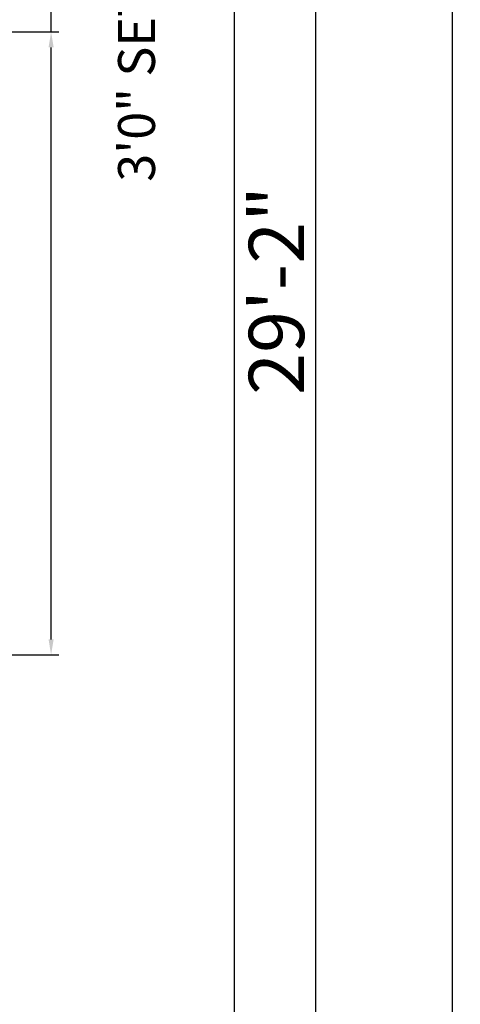
# Model space of a CAD drawing. Units: inches. Extents: x 3321 to 5237, y 11 to 1752.
# Tile 37 of 43: x 5131 to 5203, y 1396 to 1556. Entities that reach past the tile are written whole.
import ezdxf

# ---------------------------------------------------------------- set-up
doc = ezdxf.new("R2010")
doc.units = ezdxf.units.IN
for name, color, linetype, lineweight in [('A-ANNO-DIMS', 2, 'Continuous', 18), ('A-ANNO-TEXT', 7, 'Continuous', 18), ('C-PROP', 7, 'Continuous', 30)]:
    doc.layers.add(name, color=color, linetype=linetype, lineweight=lineweight)
doc.styles.get("Standard").update_dxf_attribs({"font": 'arial.ttf'})
doc.dimstyles.new('ISO-25', dxfattribs={"dimtxt": 9, "dimasz": 2.5, "dimexe": 1.25, "dimexo": 0.625, "dimtad": 1, "dimdec": 1, "dimlunit": 3, "dimtxsty": 'Standard', "dimcen": 2.5, "dimclrd": 4, "dimclre": 4, "dimclrt": 256, "dimadec": 0, "dimazin": 0, "dimtfac": 1, "dimtdec": 1, "dimtmove": 0, "dimatfit": 3, "dimfxl": 1, "dimarcsym": 0})

# ---------------------------------------------------------------- blocks, each defined once
blk = doc.blocks.new('*D22')
at = {"layer": 'A-ANNO-DIMS', "color": 0, "lineweight": -2, "transparency": 16777216}
for p, q in [((5166.71, 1687.34), (5180.54, 1687.34)), ((5179.29, 1339.84), (5179.29, 1684.84)), ((5166.71, 1337.34), (5180.54, 1337.34))]:
    blk.add_line(p, q, dxfattribs=at)
at = {"layer": 'A-ANNO-DIMS', "color": 0, "transparency": 16777216}
for points in [[(5178.88, 1684.84), (5179.71, 1684.84), (5179.29, 1687.34)], [(5178.88, 1339.84), (5179.71, 1339.84), (5179.29, 1337.34)]]:
    blk.add_solid(points, dxfattribs=at)
at = {"layer": 'Defpoints', "color": 0, "transparency": 16777216}
for p in [(5166.08, 1687.34), (5179.29, 1687.34), (5166.08, 1337.34)]:
    blk.add_point(p, dxfattribs=at)
at = {"layer": 'A-ANNO-DIMS', "color": 0, "transparency": 16777216, "insert": (5174.07, 1512.34), "char_height": 9, "attachment_point": 5, "rotation": 90}
blk.add_mtext('29\'-2"', dxfattribs=at)
blk = doc.blocks.new('*D148')
at = {"layer": 'A-ANNO-DIMS', "color": 0, "lineweight": -2, "transparency": 16777216}
for p, q in [((5166.71, 1707.34), (5202.79, 1707.34)), ((5201.54, 989.84), (5201.54, 1704.84)), ((5166.71, 987.34), (5202.79, 987.34))]:
    blk.add_line(p, q, dxfattribs=at)
at = {"layer": 'A-ANNO-DIMS', "color": 0, "transparency": 16777216}
for points in [[(5201.12, 1704.84), (5201.96, 1704.84), (5201.54, 1707.34)], [(5201.12, 989.84), (5201.96, 989.84), (5201.54, 987.34)]]:
    blk.add_solid(points, dxfattribs=at)
at = {"layer": 'Defpoints', "color": 0, "transparency": 16777216}
for p in [(5166.08, 1707.34), (5201.54, 1707.34), (5166.08, 987.34)]:
    blk.add_point(p, dxfattribs=at)
at = {"layer": 'A-ANNO-DIMS', "color": 0, "transparency": 16777216, "insert": (5196.32, 1347.34), "char_height": 9, "attachment_point": 5, "rotation": 90}
blk.add_mtext("60'", dxfattribs=at)
blk = doc.blocks.new('PROPERTY-40X60FT')
blk.add_line((0, 720), (0, 0))
blk = doc.blocks.new('*D193')
at = {"layer": 'A-ANNO-DIMS', "color": 4, "lineweight": -2, "transparency": 16777216}
for p, q in [((5136.26, 1554.34), (5136.26, 1691.49)), ((5121.71, 1554.34), (5137.51, 1554.34)), ((5136.26, 1455.64), (5136.26, 1551.84)), ((5121.71, 1453.14), (5137.51, 1453.14))]:
    blk.add_line(p, q, dxfattribs=at)
at = {"layer": 'A-ANNO-DIMS', "color": 4, "transparency": 16777216}
for points in [[(5135.85, 1551.84), (5136.68, 1551.84), (5136.26, 1554.34)], [(5135.85, 1455.64), (5136.68, 1455.64), (5136.26, 1453.14)]]:
    blk.add_solid(points, dxfattribs=at)
at = {"layer": 'Defpoints', "color": 0, "transparency": 16777216}
for p in [(5121.08, 1554.34), (5136.26, 1554.34), (5121.08, 1453.14)]:
    blk.add_point(p, dxfattribs=at)
at = {"layer": 'A-ANNO-DIMS', "transparency": 16777216, "insert": (5130.98, 1624.17), "char_height": 9, "attachment_point": 5, "rotation": 90}
blk.add_mtext('BED GROUP 8\'-5" TYP.', dxfattribs=at)
blk = doc.blocks.new('*D197')
at = {"layer": 'A-ANNO-DIMS', "color": 4, "lineweight": -2, "transparency": 16777216}
for p, q in [((5117.01, 1364.83), (5117.01, 1476.21)), ((5114.11, 1364.83), (5118.26, 1364.83)), ((5117.01, 1343.84), (5117.01, 1362.33)), ((5114.11, 1341.34), (5118.26, 1341.34))]:
    blk.add_line(p, q, dxfattribs=at)
at = {"layer": 'A-ANNO-DIMS', "color": 4, "transparency": 16777216}
for points in [[(5116.59, 1362.33), (5117.43, 1362.33), (5117.01, 1364.83)], [(5116.59, 1343.84), (5117.43, 1343.84), (5117.01, 1341.34)]]:
    blk.add_solid(points, dxfattribs=at)
at = {"layer": 'Defpoints', "color": 0, "transparency": 16777216}
for p in [(5113.49, 1364.83), (5117.01, 1364.83), (5113.49, 1341.34)]:
    blk.add_point(p, dxfattribs=at)
at = {"layer": 'A-ANNO-DIMS', "transparency": 16777216, "insert": (5111.73, 1421.77), "char_height": 9, "attachment_point": 5, "rotation": 90}
blk.add_mtext('WC 1\'-11 1/2" TYP.', dxfattribs=at)

msp = doc.modelspace()

# ---------------------------------------------------------------- block references
at = {"layer": 'C-PROP', "rotation": 180}
msp.add_blockref('PROPERTY-40X60FT', (5166.08, 1707.34), dxfattribs=at)

# ---------------------------------------------------------------- texts
at = {"layer": 'A-ANNO-TEXT', "insert": (5147.15, 1530.01), "char_height": 6, "attachment_point": 1, "rotation": 90}
msp.add_mtext_dynamic_manual_height_columns('3\'0" SETBACK', width=97.3114, gutter_width=25, heights=[0], dxfattribs=at)

# ---------------------------------------------------------------- dimensions: what is measured, and where the dimension line sits
at = {"layer": 'A-ANNO-DIMS'}
for base, p1, p2, angle, override, picture, middle in [((5201.54, 1707.34), (5166.08, 987.34), (5166.08, 1707.34), 270, {"dimclrd": 0, "dimclre": 0, "dimclrt": 0}, '*D148', (5196.32, 1347.34)), ((5179.29, 1687.34), (5166.08, 1337.34), (5166.08, 1687.34), 90, {"dimclrd": 0, "dimclre": 0, "dimclrt": 0, "dimtmove": 1}, '*D22', (5174.07, 1512.34))]:
    dim = msp.add_linear_dim(base=base, p1=p1, p2=p2, angle=angle, dimstyle='ISO-25', override=override, dxfattribs=at)
    dim.commit()
    dim.dimension.update_dxf_attribs({"geometry": picture, "text_midpoint": middle})
for base, p1, p2, text, picture, middle in [((5136.26, 1554.34), (5121.08, 1453.14), (5121.08, 1554.34), 'BED GROUP <> TYP.', '*D193', (5130.98, 1624.17)), ((5117.01, 1364.83), (5113.49, 1341.34), (5113.49, 1364.83), 'WC <> TYP.', '*D197', (5111.73, 1421.77))]:
    dim = msp.add_linear_dim(base=base, p1=p1, p2=p2, angle=90, text=text, dimstyle='ISO-25', override={"dimdec": 1, "dimlfac": 1, "dimrnd": 0, "dimzin": 1, "dimdsep": 46, "dimlunit": 4, "dimfrac": 2}, dxfattribs=at)
    dim.commit()
    dim.dimension.update_dxf_attribs({"geometry": picture, "text_midpoint": middle})

doc.saveas('drawing.dxf')
